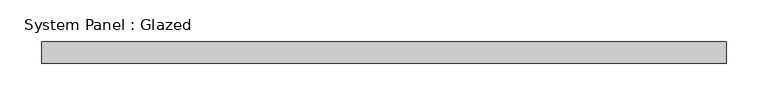
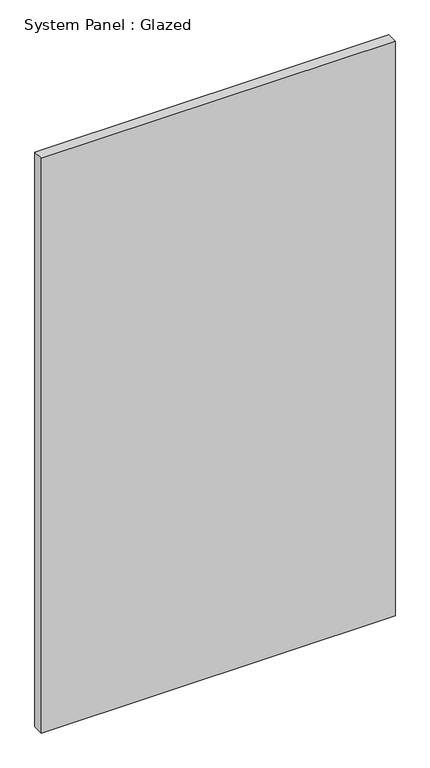
"""IFC4 building model written with IfcOpenShell, lengths in millimetres: plate geometry, System Panel : Glazed."""

from ifc_helpers import new_model, si_unit, origin, origin_with_axes, place, context, project, spatial, polyline, outline, extrude, source, transform, mapped, element, save


def system_panel_glazed_a910ef8c(model_context):
    return source(origin(), model_context, "Body", "SweptSolid", [
        extrude(outline(polyline([(409.575, 19.05), (-409.575, 19.05), (-409.575, 44.45), (409.575, 44.45), (409.575, 19.05)])), origin_with_axes(), (0.0, 0.0, 1.0), 1406.754744),
    ])


if __name__ == "__main__":
    model = new_model("IFC4")
    model_context = context("Model", 3, world=origin())
    ifc_project = project(units=[si_unit("LENGTHUNIT", "METRE", prefix="MILLI")], contexts=[model_context])
    site = spatial("IfcSite", under=ifc_project)
    building = spatial("IfcBuilding", under=site)
    placement = place(None, origin())
    system_panel_glazed_shape = system_panel_glazed_a910ef8c(model_context)
    element("IfcPlate", 1, ObjectType="System Panel : Glazed", at=placement, inside=building, context=model_context, shape_type="MappedRepresentation", body=[
        mapped(system_panel_glazed_shape, transform((0.0, 0.0, 0.0), x_axis=(1.0, 0.0, 0.0), y_axis=(0.0, 1.0, 0.0), z_axis=(0.0, 0.0, 1.0))),
    ])
    save(model, "model.ifc")

# Revit data of these elements
# Type "System Panel : Glazed"
#   Construction Type Id = "GSP4R"
#   Analytic Construction = "1/8 in Pilkington single glazing"
#   Visual Light Transmittance = 0.9
#   Solar Heat Gain Coefficient = 0.86
#   Heat Transfer Coefficient (U) = 1.18115 BTU/(h·ft²·°F)
#   Define Thermal Properties by = 1
# Element 1 (IfcPlate, "System Panel : Glazed")
#   Materials on its faces: "Glass"
# Materials
#   "Glass": class "Glass", colour RGB 0 128 192, transparency 0.75, Description = "Soda Lime Glass", Cost = 0
